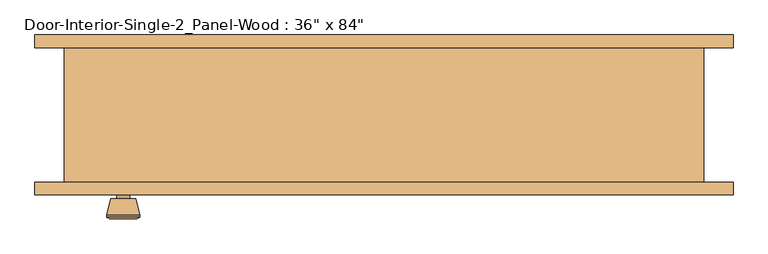
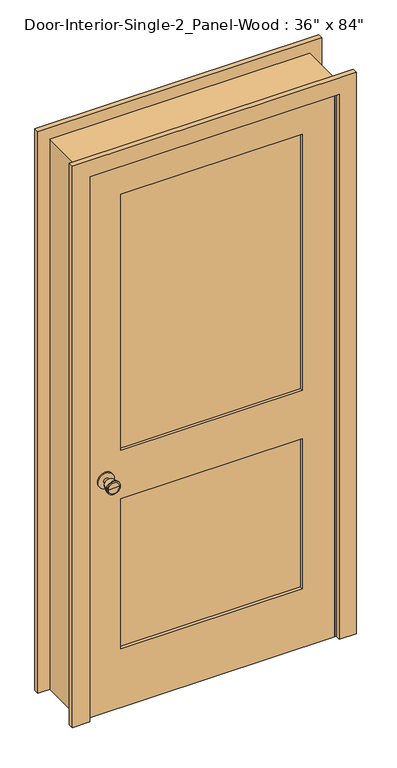
"""IFC4 building model written with IfcOpenShell, lengths in millimetres: door geometry."""

from ifc_helpers import new_model, si_unit, point, frame, frame_2d, origin, place, context, project, spatial, polyline, circle_curve, trimmed, segment, composite_curve, outline, extrude, faceted_brep, source, transform, mapped, element, save
from ifc_brep_helpers import plane_surface, cylinder_surface, revolved_surface, advanced_brep


def door_387d6dd4(model_context):
    return source(origin(), model_context, "Body", "SolidModel", [
        advanced_brep(
        [(-393.7, -57.5, 914.4), (-403.7, -57.5, 914.4), (-383.7, -57.5, 914.4), (-373.2241324, -8.5, 914.4), (-414.1758676, -8.5, 914.4), (-393.7, -8.5, 914.4), (-368.7, -10.3278681, 914.4), (-418.7, -10.3278681, 914.4), (-368.7, -13.7915463, 914.4), (-418.7, -13.7915463, 914.4), (-375.063764, -38.5, 914.4), (-412.336236, -38.5, 914.4), (-383.7, -38.5, 914.4), (-403.7, -38.5, 914.4)],
        [
            (0, 1),
            (1, 2, circle_curve(frame((-393.7, -57.5, 914.4), z_axis=(0.0, -1.0, 0.0), x_axis=(-1.0, 0.0, 0.0)), 10.0)),
            (2, 0),
            (2, 1, circle_curve(frame((-393.7, -57.5, 914.4), z_axis=(0.0, -1.0, 0.0), x_axis=(-1.0, 0.0, 0.0)), 10.0)),
            (3, 4, circle_curve(frame((-393.7, -8.5, 914.4), z_axis=(0.0, 1.0, 0.0), x_axis=(-1.0, 0.0, 0.0)), 20.4758676)),
            (4, 5),
            (5, 3),
            (4, 3, circle_curve(frame((-393.7, -8.5, 914.4), z_axis=(0.0, 1.0, 0.0), x_axis=(-1.0, 0.0, 0.0)), 20.4758676)),
            (6, 7, circle_curve(frame((-393.7, -10.3278681, 914.4), z_axis=(0.0, 1.0, 0.0), x_axis=(-1.0, 0.0, 0.0)), 25.0)),
            (7, 4),
            (3, 6),
            (7, 6, circle_curve(frame((-393.7, -10.3278681, 914.4), z_axis=(0.0, 1.0, 0.0), x_axis=(-1.0, 0.0, 0.0)), 25.0)),
            (8, 9, circle_curve(frame((-393.7, -13.7915463, 914.4), z_axis=(0.0, 1.0, 0.0), x_axis=(-1.0, 0.0, 0.0)), 25.0)),
            (9, 7),
            (6, 8),
            (9, 8, circle_curve(frame((-393.7, -13.7915463, 914.4), z_axis=(0.0, 1.0, 0.0), x_axis=(-1.0, 0.0, 0.0)), 25.0)),
            (10, 11, circle_curve(frame((-393.7, -38.5, 914.4), z_axis=(0.0, 1.0, 0.0), x_axis=(-1.0, 0.0, 0.0)), 18.636236)),
            (11, 9),
            (8, 10),
            (11, 10, circle_curve(frame((-393.7, -38.5, 914.4), z_axis=(0.0, 1.0, 0.0), x_axis=(-1.0, 0.0, 0.0)), 18.636236)),
            (12, 13, circle_curve(frame((-393.7, -38.5, 914.4), z_axis=(0.0, 1.0, 0.0), x_axis=(-1.0, 0.0, 0.0)), 10.0)),
            (13, 11),
            (10, 12),
            (13, 12, circle_curve(frame((-393.7, -38.5, 914.4), z_axis=(0.0, 1.0, 0.0), x_axis=(-1.0, 0.0, 0.0)), 10.0)),
            (1, 13),
            (12, 2),
        ],
        [
            plane_surface(frame((-393.7, -57.5, 914.4), z_axis=(0.0, -1.0, 0.0), x_axis=(-1.0, 0.0, 0.0))),
            plane_surface(frame((-393.7, -8.5, 914.4), z_axis=(0.0, 1.0, 0.0), x_axis=(-1.0, 0.0, 0.0))),
            revolved_surface(polyline([(-414.1758676, -8.5, 914.4), (-418.7, -10.3278681, 914.4)]), (-393.7, -57.5, 914.4), (0.0, -1.0, 0.0)),
            cylinder_surface(frame((-393.7, -57.5, 914.4), z_axis=(0.0, -1.0, 0.0), x_axis=(-1.0, 0.0, 0.0)), 25.0),
            revolved_surface(polyline([(-418.7, -13.7915463, 914.4), (-412.336236, -38.5, 914.4)]), (-393.7, -57.5, 914.4), (0.0, -1.0, 0.0)),
            plane_surface(frame((-393.7, -38.5, 914.4), z_axis=(0.0, -1.0, 0.0), x_axis=(-1.0, 0.0, 0.0))),
            cylinder_surface(frame((-393.7, -57.5, 914.4), z_axis=(0.0, -1.0, 0.0), x_axis=(-1.0, 0.0, 0.0)), 10.0),
        ],
        [
            (0, [[1, 2, 3]]),
            (0, [[-3, 4, -1]]),
            (1, [[5, 6, 7]]),
            (1, [[8, -7, -6]]),
            (2, [[9, 10, -5, 11]]),
            (2, [[12, -11, -8, -10]]),
            (3, [[13, 14, -9, 15]]),
            (3, [[16, -15, -12, -14]]),
            (4, [[17, 18, -13, 19]]),
            (4, [[20, -19, -16, -18]]),
            (5, [[21, 22, -17, 23]]),
            (5, [[24, -23, -20, -22]]),
            (6, [[-2, 25, -21, 26]]),
            (6, [[-4, -26, -24, -25]]),
        ],
    ),
        extrude(outline(composite_curve([segment(trimmed(circle_curve(frame_2d((914.4, -393.7)), 30.0), [point((914.4, -423.7))], [point((914.4, -363.7))], False, "CARTESIAN"), True, "CONTINUOUS"), segment(trimmed(circle_curve(frame_2d((914.4, -393.7)), 30.0), [point((914.4, -363.7))], [point((914.4, -423.7))], False, "CARTESIAN"), True, "CONTINUOUS")], self_intersect=False)), frame((0.0, -63.5, 0.0), z_axis=(0.0, 1.0, 0.0), x_axis=(0.0, 0.0, 1.0)), (0.0, 0.0, 1.0), 6.0),
        advanced_brep(
        [(-393.7, -104.425, 914.4), (-383.7, -104.425, 914.4), (-403.7, -104.425, 914.4), (-373.2241324, -153.425, 914.4), (-393.7, -153.425, 914.4), (-414.1758676, -153.425, 914.4), (-368.7, -151.5971319, 914.4), (-418.7, -151.5971319, 914.4), (-368.7, -148.1334537, 914.4), (-418.7, -148.1334537, 914.4), (-375.063764, -123.425, 914.4), (-412.336236, -123.425, 914.4), (-383.7, -123.425, 914.4), (-403.7, -123.425, 914.4)],
        [
            (0, 1),
            (1, 2, circle_curve(frame((-393.7, -104.425, 914.4), z_axis=(0.0, 1.0, 0.0), x_axis=(-1.0, 0.0, 0.0)), 10.0)),
            (2, 0),
            (2, 1, circle_curve(frame((-393.7, -104.425, 914.4), z_axis=(0.0, 1.0, 0.0), x_axis=(-1.0, 0.0, 0.0)), 10.0)),
            (3, 4),
            (4, 5),
            (5, 3, circle_curve(frame((-393.7, -153.425, 914.4), z_axis=(0.0, -1.0, 0.0), x_axis=(-1.0, 0.0, 0.0)), 20.4758676)),
            (3, 5, circle_curve(frame((-393.7, -153.425, 914.4), z_axis=(0.0, -1.0, 0.0), x_axis=(-1.0, 0.0, 0.0)), 20.4758676)),
            (6, 3),
            (5, 7),
            (7, 6, circle_curve(frame((-393.7, -151.5971319, 914.4), z_axis=(0.0, -1.0, 0.0), x_axis=(-1.0, 0.0, 0.0)), 25.0)),
            (6, 7, circle_curve(frame((-393.7, -151.5971319, 914.4), z_axis=(0.0, -1.0, 0.0), x_axis=(-1.0, 0.0, 0.0)), 25.0)),
            (8, 6),
            (7, 9),
            (9, 8, circle_curve(frame((-393.7, -148.1334537, 914.4), z_axis=(0.0, -1.0, 0.0), x_axis=(-1.0, 0.0, 0.0)), 25.0)),
            (8, 9, circle_curve(frame((-393.7, -148.1334537, 914.4), z_axis=(0.0, -1.0, 0.0), x_axis=(-1.0, 0.0, 0.0)), 25.0)),
            (10, 8),
            (9, 11),
            (11, 10, circle_curve(frame((-393.7, -123.425, 914.4), z_axis=(0.0, -1.0, 0.0), x_axis=(-1.0, 0.0, 0.0)), 18.636236)),
            (10, 11, circle_curve(frame((-393.7, -123.425, 914.4), z_axis=(0.0, -1.0, 0.0), x_axis=(-1.0, 0.0, 0.0)), 18.636236)),
            (12, 10),
            (11, 13),
            (13, 12, circle_curve(frame((-393.7, -123.425, 914.4), z_axis=(0.0, -1.0, 0.0), x_axis=(-1.0, 0.0, 0.0)), 10.0)),
            (12, 13, circle_curve(frame((-393.7, -123.425, 914.4), z_axis=(0.0, -1.0, 0.0), x_axis=(-1.0, 0.0, 0.0)), 10.0)),
            (1, 12),
            (13, 2),
        ],
        [
            plane_surface(frame((-393.7, -104.425, 914.4), z_axis=(0.0, 1.0, 0.0), x_axis=(-1.0, 0.0, 0.0))),
            plane_surface(frame((-393.7, -153.425, 914.4), z_axis=(0.0, -1.0, 0.0), x_axis=(-1.0, 0.0, 0.0))),
            revolved_surface(polyline([(-414.1758676, -153.425, 914.4), (-418.7, -151.5971319, 914.4)]), (-393.7, -104.425, 914.4), (0.0, 1.0, 0.0)),
            cylinder_surface(frame((-393.7, -104.425, 914.4), z_axis=(0.0, 1.0, 0.0), x_axis=(-1.0, 0.0, 0.0)), 25.0),
            revolved_surface(polyline([(-418.7, -148.1334537, 914.4), (-412.336236, -123.425, 914.4)]), (-393.7, -104.425, 914.4), (0.0, 1.0, 0.0)),
            plane_surface(frame((-393.7, -123.425, 914.4), z_axis=(0.0, 1.0, 0.0), x_axis=(-1.0, 0.0, 0.0))),
            cylinder_surface(frame((-393.7, -104.425, 914.4), z_axis=(0.0, 1.0, 0.0), x_axis=(-1.0, 0.0, 0.0)), 10.0),
        ],
        [
            (0, [[1, 2, 3]]),
            (0, [[-3, 4, -1]]),
            (1, [[5, 6, 7]]),
            (1, [[-6, -5, 8]]),
            (2, [[9, -7, 10, 11]]),
            (2, [[-10, -8, -9, 12]]),
            (3, [[13, -11, 14, 15]]),
            (3, [[-14, -12, -13, 16]]),
            (4, [[17, -15, 18, 19]]),
            (4, [[-18, -16, -17, 20]]),
            (5, [[21, -19, 22, 23]]),
            (5, [[-22, -20, -21, 24]]),
            (6, [[25, -23, 26, -2]]),
            (6, [[-26, -24, -25, -4]]),
        ],
    ),
        extrude(outline(composite_curve([segment(trimmed(circle_curve(frame_2d((914.4, -393.7)), 30.0), [point((914.4, -423.7))], [point((914.4, -363.7))], False, "CARTESIAN"), True, "CONTINUOUS"), segment(trimmed(circle_curve(frame_2d((914.4, -393.7)), 30.0), [point((914.4, -363.7))], [point((914.4, -423.7))], False, "CARTESIAN"), True, "CONTINUOUS")], self_intersect=False)), frame((0.0, -104.425, 0.0), z_axis=(0.0, 1.0, 0.0), x_axis=(0.0, 0.0, 1.0)), (0.0, 0.0, 1.0), 6.0),
        extrude(outline(polyline([(336.55, -75.1416667), (336.55, -86.7833333), (-336.55, -86.7833333), (-336.55, -75.1416667), (336.55, -75.1416667)])), frame((0.0, 0.0, 1009.65), z_axis=(0.0, 0.0, 1.0), x_axis=(1.0, 0.0, 0.0)), (0.0, 0.0, 1.0), 1004.8875),
        extrude(outline(polyline([(336.55, -75.1416667), (336.55, -86.7833333), (-336.55, -86.7833333), (-336.55, -75.1416667), (336.55, -75.1416667)])), frame((0.0, 0.0, 231.775), z_axis=(0.0, 0.0, 1.0), x_axis=(1.0, 0.0, 0.0)), (0.0, 0.0, 1.0), 587.375),
        extrude(outline(polyline([(2133.6, -457.2), (0.0, -457.2), (0.0, 457.2), (2133.6, 457.2), (2133.6, -457.2)]), holes=[polyline([(2014.5375, -336.55), (2014.5375, 336.55), (1009.65, 336.55), (1009.65, -336.55), (2014.5375, -336.55)]), polyline([(819.15, -336.55), (819.15, 336.55), (231.775, 336.55), (231.775, -336.55), (819.15, -336.55)])]), frame((0.0, -98.425, 0.0), z_axis=(0.0, 1.0, 0.0), x_axis=(0.0, 0.0, 1.0)), (0.0, 0.0, 1.0), 34.925),
        faceted_brep([(482.6, -98.425, 0.0), (457.2, -98.425, 0.0), (457.2, -63.5, 0.0), (444.5, -63.5, 0.0), (444.5, -28.575, 0.0), (457.2, -28.575, 0.0), (457.2, 104.775, 0.0), (482.6, 104.775, 0.0), (482.6, 104.775, 2159.0), (482.6, -98.425, 2159.0), (457.2, 104.775, 2133.6), (-457.2, 104.775, 2133.6), (-457.2, 104.775, 0.0), (-482.6, 104.775, 0.0), (-482.6, 104.775, 2159.0), (457.2, -28.575, 2133.6), (444.5, -28.575, 2120.9), (-444.5, -28.575, 2120.9), (-444.5, -28.575, 0.0), (-457.2, -28.575, 0.0), (-457.2, -28.575, 2133.6), (444.5, -63.5, 2120.9), (457.2, -63.5, 2133.6), (-457.2, -63.5, 2133.6), (-457.2, -63.5, 0.0), (-444.5, -63.5, 0.0), (-444.5, -63.5, 2120.9), (457.2, -98.425, 2133.6), (-482.6, -98.425, 2159.0), (-482.6, -98.425, 0.0), (-457.2, -98.425, 0.0), (-457.2, -98.425, 2133.6)], [[[0, 1, 2, 3, 4, 5, 6, 7]], [[7, 8, 9, 0]], [[6, 10, 11, 12, 13, 14, 8, 7]], [[5, 15, 10, 6]], [[4, 16, 17, 18, 19, 20, 15, 5]], [[3, 21, 16, 4]], [[2, 22, 23, 24, 25, 26, 21, 3]], [[1, 27, 22, 2]], [[0, 9, 28, 29, 30, 31, 27, 1]], [[8, 14, 28, 9]], [[15, 20, 11, 10]], [[21, 26, 17, 16]], [[27, 31, 23, 22]], [[29, 13, 12, 19, 18, 25, 24, 30]], [[14, 13, 29, 28]], [[20, 19, 12, 11]], [[26, 25, 18, 17]], [[31, 30, 24, 23]]]),
        extrude(outline(polyline([(0.0, 527.05), (2203.45, 527.05), (2203.45, -527.05), (0.0, -527.05), (0.0, -463.55), (2139.95, -463.55), (2139.95, 463.55), (0.0, 463.55), (0.0, 527.05)])), frame((0.0, 104.775, 0.0), z_axis=(0.0, 1.0, 0.0), x_axis=(0.0, 0.0, 1.0)), (0.0, 0.0, 1.0), 19.05),
        extrude(outline(polyline([(0.0, 527.05), (2203.45, 527.05), (2203.45, -527.05), (0.0, -527.05), (0.0, -463.55), (2139.95, -463.55), (2139.95, 463.55), (0.0, 463.55), (0.0, 527.05)])), frame((0.0, -117.475, 0.0), z_axis=(0.0, 1.0, 0.0), x_axis=(0.0, 0.0, 1.0)), (0.0, 0.0, 1.0), 19.05),
    ])


if __name__ == "__main__":
    model = new_model("IFC4")
    model_context = context("Model", 3, world=origin())
    ifc_project = project(units=[si_unit("LENGTHUNIT", "METRE", prefix="MILLI")], contexts=[model_context])
    site = spatial("IfcSite", under=ifc_project)
    building = spatial("IfcBuilding", under=site)
    placement = place(None, origin())
    door_shape = door_387d6dd4(model_context)
    element("IfcDoor", 1, ObjectType="Door-Interior-Single-2_Panel-Wood : 36\" x 84\"", at=placement, inside=building, context=model_context, shape_type="MappedRepresentation", body=[
        mapped(door_shape, transform((0.0, 0.0, 0.0), x_axis=(1.0, 0.0, 0.0), y_axis=(0.0, 1.0, 0.0), z_axis=(0.0, 0.0, 1.0))),
    ])
    save(model, "model.ifc")

# Revit data of these elements
# Type "Door-Interior-Single-2_Panel-Wood : 36\" x 84\""
#   Type Mark = "9"
#   Assembly Code = "C1020300"
#   Analytic Construction = "Wooden"
#   Top Rail = 0' - 4 11/16"
#   Thickness = 0' - 1 3/8"
#   Thermal Resistance (R) = 2.5876 (h·ft²·°F)/BTU
#   Swing Angle [instance default] = 90.00°
#   Stiles = 0' - 4 3/4"
#   Rough Width = 3' - 2"
#   Rough Height = 7' - 1"
#   Lock Rail = 0' - 7 1/2"
#   Height = 7' - 0"
#   Width = 3' - 0"
#   Heat Transfer Coefficient (U) = 0.3865 BTU/(h·ft²·°F)
#   Bottom Rail = 0' - 9 1/8"
#   Trim Material = Cherry
#   Panel Material = Cherry
#   Frame Material = Cherry
#   Door Handle Material = Aluminum
#   Visual Light Transmittance = 0
#   Solar Heat Gain Coefficient = 0
#   Wall Closure = (empty or 0)
#   Function = (empty or 0)
# Element 1 (IfcDoor, "Door-Interior-Single-2_Panel-Wood : 36\" x 84\"")
#   Materials on its faces: "Cherry", "Aluminum"
# Materials
#   "Cherry": class "Wood", colour RGB 226 177 128, transparency 0, Description = "Prunus Serotina", Cost = 0
#   "Aluminum": class "Metal", colour RGB 247 247 247, transparency 0, Description = "Aluminum 6061", Cost = 0
